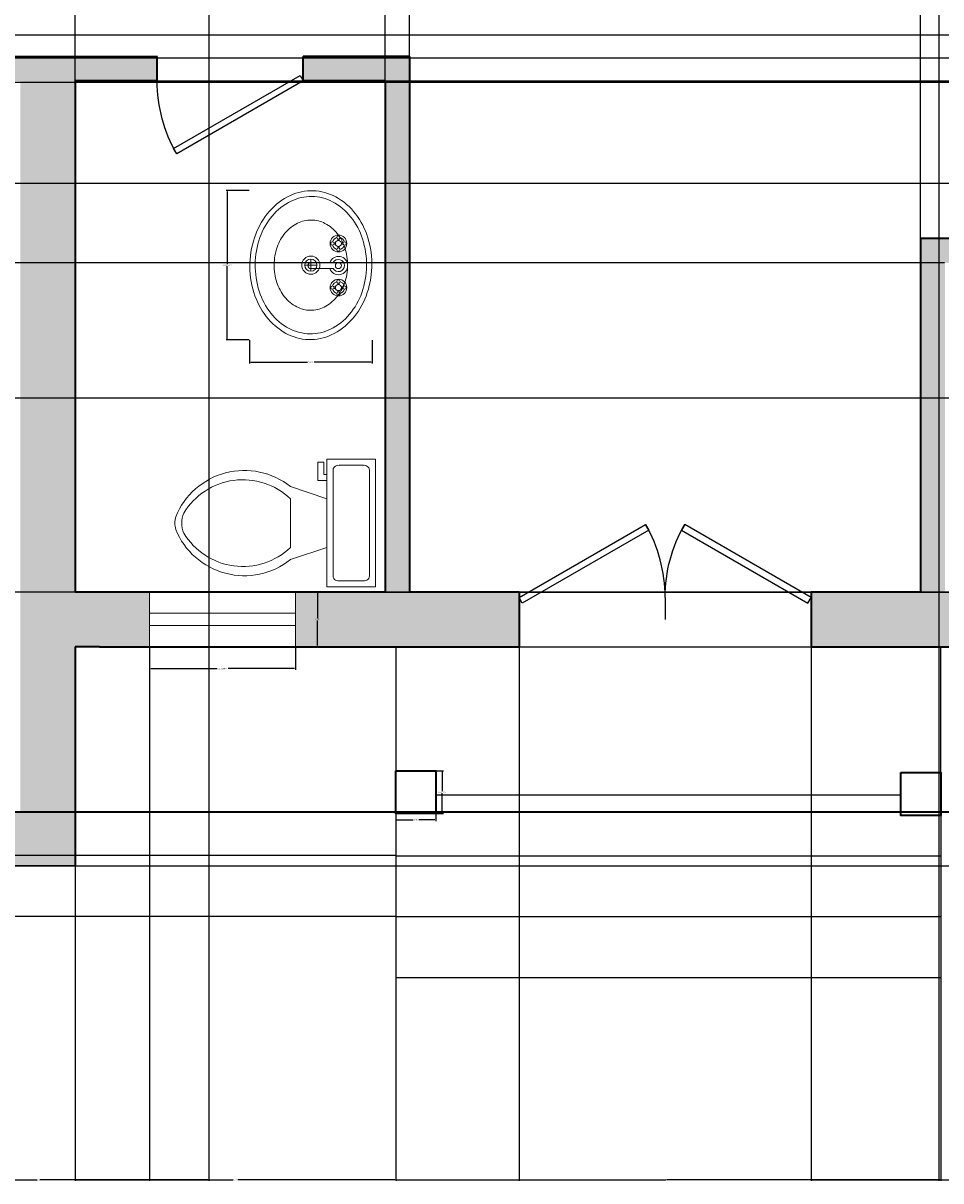
# Model space of a CAD drawing. Units: inches. Extents: x 1531 to 2263, y 2711 to 3216.
# Tile 7 of 12: x 1925 to 2076, y 2711 to 2901. Entities that reach past the tile are written whole.
import ezdxf

# ---------------------------------------------------------------- set-up
doc = ezdxf.new("R2010")
doc.units = ezdxf.units.IN
for name, color, linetype, lineweight in [('A-ANNO-DIMS', 2, 'Continuous', 18), ('A-COLS', 7, 'Continuous', 35), ('A-DOOR', 3, 'Continuous', 25), ('A-FLOR-FIXT', 9, 'Continuous', 18), ('A-FLOR-STRS', 7, 'Continuous', 25), ('A-GLAZ', 4, 'Continuous', 18), ('A-WALL', 7, 'Continuous', 35)]:
    doc.layers.add(name, color=color, linetype=linetype, lineweight=lineweight)
doc.layers.add('A-WALL-PATT', color=18, linetype='Continuous', lineweight=13, true_color=0x000000)
doc.styles.get("Standard").update_dxf_attribs({"font": 'arial.ttf'})
doc.dimstyles.get("Standard").update_dxf_attribs({"dimtxt": 0.18, "dimasz": 0.18, "dimexe": 0.18, "dimexo": 0.0625, "dimgap": 0.09, "dimtad": 0, "dimtih": 1, "dimtoh": 1, "dimdec": 4, "dimzin": 0, "dimdsep": 46, "dimtxsty": 'Standard', "dimcen": 0.09, "dimadec": 0, "dimazin": 0, "dimtfac": 1, "dimtdec": 4, "dimtofl": 0, "dimtmove": 0, "dimatfit": 3, "dimfxl": 1, "dimtolj": 1, "dimtzin": 0, "dimarcsym": 0})

# ---------------------------------------------------------------- blocks, each defined once
blk = doc.blocks.new('*U3')
for p, q in [((0, 0), (0, -6)), ((40, 0), (40, -6))]:
    blk.add_line(p, q)
blk.add_lwpolyline([(0, 0), (34.64, 20), (35.52, 18.48), (0.87, -1.52)], close=True)
blk.add_arc((0, 0), 40, 0, 30)
blk = doc.blocks.new('*U6')
for p, q in [((0, 0), (0, 6)), ((40, 0), (40, 6))]:
    blk.add_line(p, q)
blk.add_lwpolyline([(0, 0), (34.64, -20), (35.52, -18.48), (0.87, 1.52)], close=True)
blk.add_arc((0, 0), 40, 330, 0)
blk = doc.blocks.new('Toilet - top')
for p, q in [((9.5, -6), (9.5, -2)), ((-10, -8.5), (-8, -8.5)), ((-10, -9.5), (-10, -8.5)), ((-7, -9.5), (-10, -9.5)), ((-8, -8.5), (-8, -8)), ((-7, -8), (-7, -9.5)), ((-4, -8), (-6, -14)), ((4, -8), (6, -14)), ((4, -14), (-4, -14))]:
    blk.add_line(p, q)
blk.add_lwpolyline([(10.5, -8), (10.5, 0), (-10.5, 0), (-10.5, -8)], close=True)
for points in [[(8.5, -1), (-8.5, -1)], [(-9.5, -2), (-9.5, -6)], [(-8.5, -7), (8.5, -7)]]:
    blk.add_lwpolyline(points)
for centre, radius, start, end in [((-8.62, -1.88), 0.884, 81.8699, 188.1301), ((8.62, -1.88), 0.884, 351.8699, 98.1301), ((-8.62, -6.12), 0.884, 171.8699, 278.1301), ((8.62, -6.12), 0.884, 261.8699, 8.1301), ((3.52, -21.58), 12.17, 141.4691, 247.9714), ((4.2, -21.82), 11.33, 136.3677, 238.9468), ((-3.52, -21.58), 12.17, 292.0284, 38.5307), ((-4.2, -21.82), 11.33, 301.053, 43.6321), ((0, -27.88), 4, 245.7318, 294.2682), ((0, -29), 4, 254.8605, 285.1395)]:
    blk.add_arc(centre, radius, start, end)
blk = doc.blocks.new('Sink - Oval top')
for p, q in [((-1, 0), (1, 0)), ((0, 1), (0, -1))]:
    blk.add_line(p, q)
for points in [[(-12.23, 0.39, 0.117634), (-11.46, -3.36, 0.104469), (-8.88, -6.8, 0.090016), (-5.08, -9.07, 0.08192), (-0.32, -10.02, 0.08192), (4.49, -9.38, 0.090016), (8.42, -7.36, 0.104469), (11.22, -4.09, 0.117634), (12.23, -0.39, 0.117634), (11.46, 3.36, 0.104469), (8.88, 6.8, 0.090016), (5.08, 9.07, 0.08192), (0.32, 10.02, 0.08192), (-4.49, 9.38, 0.090016), (-8.42, 7.36, 0.104469), (-11.22, 4.09, 0.117634)], [(-11.29, 0.16, 0.118622), (-10.52, -3.25, 0.104678), (-8.07, -6.36, 0.089562), (-4.54, -8.37, 0.081185), (-0.13, -9.15, 0.081185), (4.3, -8.49, 0.089562), (7.89, -6.58, 0.104678), (10.42, -3.55, 0.118622), (11.29, -0.16, 0.118622), (10.52, 3.25, 0.104678), (8.07, 6.36, 0.089562), (4.54, 8.37, 0.081185), (0.13, 9.15, 0.081185), (-4.3, 8.49, 0.089562), (-7.89, 6.58, 0.104678), (-10.42, 3.55, 0.118622)], [(-7.42, 0.08, 0.118283), (-6.91, -2.17, 0.104607), (-5.29, -4.21, 0.089718), (-2.97, -5.53, 0.081436), (-0.07, -6.04, 0.081436), (2.84, -5.59, 0.089718), (5.2, -4.33, 0.104607), (6.86, -2.32, 0.118283), (7.42, -0.08, 0.118283), (6.91, 2.17, 0.104607), (5.29, 4.21, 0.089718), (2.97, 5.53, 0.081436), (0.07, 6.04, 0.081436), (-2.84, 5.59, 0.089718), (-5.2, 4.33, 0.104607), (-6.86, 2.32, 0.118283)]]:
    blk.add_lwpolyline(points, format="xyb", close=True)
for radius in [1.5, 1]:
    blk.add_circle((0, 0), radius)
blk = doc.blocks.new('Faucet - Bathroom top')
for p, q in [((-4.107, 0.125), (-4.375, 0.125)), ((-3.75, 0.4788), (-3.75, 0.75)), ((-3.5, 0.482), (-3.5, 0.75)), ((-3.1461, 0.125), (-2.875, 0.125)), ((3.143, 0.125), (2.875, 0.125)), ((3.5, 0.4788), (3.5, 0.75)), ((3.75, 0.482), (3.75, 0.75)), ((4.1039, 0.125), (4.375, 0.125)), ((-4.1039, -0.125), (-4.375, -0.125)), ((-3.75, -0.4821), (-3.75, -0.75)), ((-3.5, -0.4789), (-3.5, -0.75)), ((-3.143, -0.125), (-2.875, -0.125)), ((-0.5, -0.8639), (-0.5, -4.5)), ((0.5, -4.5), (0.5, -0.8631)), ((3.1461, -0.125), (2.875, -0.125)), ((3.5, -0.4821), (3.5, -0.75)), ((3.75, -0.4789), (3.75, -0.75)), ((4.107, -0.125), (4.375, -0.125))]:
    blk.add_line(p, q)
for centre, radius in [((-3.625, 0), 1.375), ((-4.625, 0), 0.2795), ((-3.625, 0), 0.5), ((-3.625, 1), 0.2795), ((-2.625, 0), 0.2795), ((0, 0), 0.5), ((3.625, 0), 1.375), ((2.625, 0), 0.2795), ((3.625, 0), 0.5), ((3.625, 1), 0.2795), ((4.625, 0), 0.2795), ((-3.625, -1), 0.2795), ((3.625, -1), 0.2795)]:
    blk.add_circle(centre, radius)
for centre, radius, start, end in [((-3.625, 0), 1, 105.2407, 164.2093), ((-3.625, 0), 1, 16.44125, 74.07887), ((0, 0), 1.5, 289.6514, 250.3603), ((0, 0), 1, 300.3431, 239.7554), ((3.625, 0), 1, 106.12, 164.0884), ((3.625, 0), 1, 16.23422, 73.90469), ((-3.625, 0), 1, 196.2342, 253.9047), ((-3.625, 0), 1, 286.12, 344.0884), ((3.625, 0), 1, 196.4413, 254.0789), ((3.625, 0), 1, 285.2407, 344.2093), ((0, -4.5), 0.5, 180, 0)]:
    blk.add_arc(centre, radius, start, end)
blk = doc.blocks.new('WIN-24IN')
for p, q in [((0, 5.5), (24, 5.5)), ((0, 3.5), (24, 3.5))]:
    blk.add_line(p, q)
for points in [[(0, 9), (0, 0)], [(24, 0), (24, 9)]]:
    blk.add_lwpolyline(points)
blk = doc.blocks.new('PORCH-POST')
blk.add_lwpolyline([(0, 7.03), (6.58, 7.03), (6.58, 0), (0, 0)], close=True)
blk = doc.blocks.new('*D28')
at = {"layer": 'A-ANNO-DIMS', "color": 0, "lineweight": -2, "transparency": 16777216}
for p, q in [((1946.17, 2798.8), (1946.17, 2795.08)), ((1970.17, 2798.8), (1970.17, 2795.08)), ((1946.35, 2795.26), (1957.27, 2795.26)), ((1969.99, 2795.26), (1959.06, 2795.26))]:
    blk.add_line(p, q, dxfattribs=at)
at = {"layer": 'A-ANNO-DIMS', "color": 0, "transparency": 16777216}
for points in [[(1946.35, 2795.29), (1946.35, 2795.23), (1946.17, 2795.26)], [(1969.99, 2795.29), (1969.99, 2795.23), (1970.17, 2795.26)]]:
    blk.add_solid(points, dxfattribs=at)
at = {"layer": 'Defpoints', "color": 0, "transparency": 16777216}
for p in [(1946.17, 2798.86), (1970.17, 2798.86), (1970.17, 2795.26)]:
    blk.add_point(p, dxfattribs=at)
at = {"layer": 'A-ANNO-DIMS', "color": 0, "transparency": 16777216, "insert": (1958.17, 2795.26), "char_height": 0.18, "attachment_point": 5}
blk.add_mtext('\\A1;WDW 24 TYP.', dxfattribs=at)
blk = doc.blocks.new('*D29')
at = {"layer": 'A-ANNO-DIMS', "color": 0, "lineweight": -2, "transparency": 16777216}
for p, q in [((1970.23, 2807.86), (1973.95, 2807.86)), ((1973.77, 2807.68), (1973.77, 2803.55)), ((1973.77, 2799.04), (1973.77, 2803.18)), ((1970.23, 2798.86), (1973.95, 2798.86))]:
    blk.add_line(p, q, dxfattribs=at)
at = {"layer": 'A-ANNO-DIMS', "color": 0, "transparency": 16777216}
for points in [[(1973.74, 2807.68), (1973.8, 2807.68), (1973.77, 2807.86)], [(1973.74, 2799.04), (1973.8, 2799.04), (1973.77, 2798.86)]]:
    blk.add_solid(points, dxfattribs=at)
at = {"layer": 'Defpoints', "color": 0, "transparency": 16777216}
for p in [(1970.17, 2807.86), (1973.77, 2807.86), (1970.17, 2798.86)]:
    blk.add_point(p, dxfattribs=at)
at = {"layer": 'A-ANNO-DIMS', "color": 0, "transparency": 16777216, "insert": (1973.77, 2803.36), "char_height": 0.18, "attachment_point": 5}
blk.add_mtext('\\A1;9 TYP.', dxfattribs=at)
blk = doc.blocks.new('*D38')
at = {"layer": 'A-ANNO-DIMS', "color": 0, "lineweight": -2, "transparency": 16777216}
for p, q in [((1962.54, 2873.87), (1958.74, 2873.87)), ((1958.92, 2873.69), (1958.92, 2861.78)), ((1958.92, 2849.5), (1958.92, 2861.41)), ((1962.54, 2849.32), (1958.74, 2849.32))]:
    blk.add_line(p, q, dxfattribs=at)
at = {"layer": 'A-ANNO-DIMS', "color": 0, "transparency": 16777216}
for points in [[(1958.89, 2873.69), (1958.95, 2873.69), (1958.92, 2873.87)], [(1958.89, 2849.5), (1958.95, 2849.5), (1958.92, 2849.32)]]:
    blk.add_solid(points, dxfattribs=at)
at = {"layer": 'Defpoints', "color": 0, "transparency": 16777216}
for p in [(1962.6, 2873.87), (1958.92, 2849.32), (1962.6, 2849.32)]:
    blk.add_point(p, dxfattribs=at)
at = {"layer": 'A-ANNO-DIMS', "color": 0, "transparency": 16777216, "insert": (1958.92, 2861.59), "char_height": 0.18, "attachment_point": 5}
blk.add_mtext('\\A1;BASIN 25 TYP.', dxfattribs=at)
blk = doc.blocks.new('*D39')
at = {"layer": 'A-ANNO-DIMS', "color": 0, "lineweight": -2, "transparency": 16777216}
for p, q in [((1962.6, 2849.25), (1962.6, 2845.45)), ((1982.74, 2849.25), (1982.74, 2845.45)), ((1962.78, 2845.63), (1972.14, 2845.63)), ((1982.56, 2845.63), (1973.2, 2845.63))]:
    blk.add_line(p, q, dxfattribs=at)
at = {"layer": 'A-ANNO-DIMS', "color": 0, "transparency": 16777216}
for points in [[(1962.78, 2845.66), (1962.78, 2845.6), (1962.6, 2845.63)], [(1982.56, 2845.66), (1982.56, 2845.6), (1982.74, 2845.63)]]:
    blk.add_solid(points, dxfattribs=at)
at = {"layer": 'Defpoints', "color": 0, "transparency": 16777216}
for p in [(1962.6, 2849.32), (1982.74, 2849.32), (1982.74, 2845.63)]:
    blk.add_point(p, dxfattribs=at)
at = {"layer": 'A-ANNO-DIMS', "color": 0, "transparency": 16777216, "insert": (1972.67, 2845.63), "char_height": 0.18, "attachment_point": 5}
blk.add_mtext('\\A1;20 TYP.', dxfattribs=at)
blk = doc.blocks.new('*D44')
at = {"layer": 'A-ANNO-DIMS', "color": 0, "lineweight": -2, "transparency": 16777216}
for p, q in [((1993.29, 2778.47), (1994.46, 2778.47)), ((1994.28, 2778.29), (1994.28, 2775.14)), ((1994.28, 2771.62), (1994.28, 2774.77)), ((1993.29, 2771.44), (1994.46, 2771.44))]:
    blk.add_line(p, q, dxfattribs=at)
at = {"layer": 'A-ANNO-DIMS', "color": 0, "transparency": 16777216}
for points in [[(1994.25, 2778.29), (1994.31, 2778.29), (1994.28, 2778.47)], [(1994.25, 2771.62), (1994.31, 2771.62), (1994.28, 2771.44)]]:
    blk.add_solid(points, dxfattribs=at)
at = {"layer": 'Defpoints', "color": 0, "transparency": 16777216}
for p in [(1993.23, 2778.47), (1994.28, 2778.47), (1993.23, 2771.44)]:
    blk.add_point(p, dxfattribs=at)
at = {"layer": 'A-ANNO-DIMS', "color": 0, "transparency": 16777216, "insert": (1994.28, 2774.96), "char_height": 0.18, "attachment_point": 5}
blk.add_mtext('\\A1;POST 7 TYP.', dxfattribs=at)
blk = doc.blocks.new('*D45')
at = {"layer": 'A-ANNO-DIMS', "color": 0, "lineweight": -2, "transparency": 16777216}
for p, q in [((1986.65, 2771.38), (1986.65, 2770.2)), ((1993.23, 2771.38), (1993.23, 2770.2)), ((1986.83, 2770.38), (1989.48, 2770.38)), ((1993.05, 2770.38), (1990.4, 2770.38))]:
    blk.add_line(p, q, dxfattribs=at)
at = {"layer": 'A-ANNO-DIMS', "color": 0, "transparency": 16777216}
for points in [[(1986.83, 2770.41), (1986.83, 2770.35), (1986.65, 2770.38)], [(1993.05, 2770.41), (1993.05, 2770.35), (1993.23, 2770.38)]]:
    blk.add_solid(points, dxfattribs=at)
at = {"layer": 'Defpoints', "color": 0, "transparency": 16777216}
for p in [(1986.65, 2771.44), (1993.23, 2771.44), (1993.23, 2770.38)]:
    blk.add_point(p, dxfattribs=at)
at = {"layer": 'A-ANNO-DIMS', "color": 0, "transparency": 16777216, "insert": (1989.94, 2770.38), "char_height": 0.18, "attachment_point": 5}
blk.add_mtext('\\A1;7 TYP.', dxfattribs=at)
blk = doc.blocks.new('*D60')
at = {"layer": 'A-ANNO-DIMS', "color": 0, "lineweight": -2, "transparency": 16777216}
for p, q in [((1899.91, 3097.79), (1899.91, 2711.06)), ((1955.91, 3097.81), (1955.91, 2711.06)), ((1900.09, 2711.24), (1927.69, 2711.24)), ((1955.73, 2711.24), (1928.13, 2711.24))]:
    blk.add_line(p, q, dxfattribs=at)
at = {"layer": 'A-ANNO-DIMS', "color": 0, "transparency": 16777216}
for points in [[(1900.09, 2711.27), (1900.09, 2711.21), (1899.91, 2711.24)], [(1955.73, 2711.27), (1955.73, 2711.21), (1955.91, 2711.24)]]:
    blk.add_solid(points, dxfattribs=at)
at = {"layer": 'Defpoints', "color": 0, "transparency": 16777216}
for p in [(1899.91, 3097.85), (1955.91, 3097.88), (1955.91, 2711.24)]:
    blk.add_point(p, dxfattribs=at)
at = {"layer": 'A-ANNO-DIMS', "color": 0, "transparency": 16777216, "insert": (1927.91, 2711.24), "char_height": 0.18, "attachment_point": 5}
blk.add_mtext('\\A1;56', dxfattribs=at)
blk = doc.blocks.new('*D65')
at = {"layer": 'A-ANNO-DIMS', "color": 0, "lineweight": -2, "transparency": 16777216}
for p, q in [((1577.97, 2891.68), (2262.37, 2891.68)), ((2262.19, 2891.5), (2262.19, 2831.86)), ((2262.19, 2771.86), (2262.19, 2831.5)), ((1577.97, 2771.68), (2262.37, 2771.68))]:
    blk.add_line(p, q, dxfattribs=at)
at = {"layer": 'A-ANNO-DIMS', "color": 0, "transparency": 16777216}
for points in [[(2262.16, 2891.5), (2262.22, 2891.5), (2262.19, 2891.68)], [(2262.16, 2771.86), (2262.22, 2771.86), (2262.19, 2771.68)]]:
    blk.add_solid(points, dxfattribs=at)
at = {"layer": 'Defpoints', "color": 0, "transparency": 16777216}
for p in [(1577.91, 2891.68), (1577.91, 2771.68), (2262.19, 2771.68)]:
    blk.add_point(p, dxfattribs=at)
at = {"layer": 'A-ANNO-DIMS', "color": 0, "transparency": 16777216, "insert": (2262.19, 2831.68), "char_height": 0.18, "attachment_point": 5}
blk.add_mtext('\\A1;120', dxfattribs=at)
blk = doc.blocks.new('*D70')
at = {"layer": 'A-ANNO-DIMS', "color": 0, "lineweight": -2, "transparency": 16777216}
for p, q in [((1736.97, 2839.76), (2262.37, 2839.76)), ((2262.19, 2839.58), (2262.19, 2805.94)), ((2262.19, 2771.94), (2262.19, 2805.58)), ((1736.97, 2771.76), (2262.37, 2771.76))]:
    blk.add_line(p, q, dxfattribs=at)
at = {"layer": 'A-ANNO-DIMS', "color": 0, "transparency": 16777216}
for points in [[(2262.16, 2839.58), (2262.22, 2839.58), (2262.19, 2839.76)], [(2262.16, 2771.94), (2262.22, 2771.94), (2262.19, 2771.76)]]:
    blk.add_solid(points, dxfattribs=at)
at = {"layer": 'Defpoints', "color": 0, "transparency": 16777216}
for p in [(1736.91, 2839.76), (2262.19, 2839.76), (1736.91, 2771.76)]:
    blk.add_point(p, dxfattribs=at)
at = {"layer": 'A-ANNO-DIMS', "color": 0, "transparency": 16777216, "insert": (2262.19, 2805.76), "char_height": 0.18, "attachment_point": 5}
blk.add_mtext('\\A1;68', dxfattribs=at)
blk = doc.blocks.new('*D71')
at = {"layer": 'A-ANNO-DIMS', "color": 0, "lineweight": -2, "transparency": 16777216}
for p, q in [((1933.91, 2891.93), (1933.91, 3216.47)), ((1934.09, 3216.29), (1959.21, 3216.29)), ((1984.73, 3216.29), (1959.61, 3216.29)), ((1984.91, 2891.95), (1984.91, 3216.47))]:
    blk.add_line(p, q, dxfattribs=at)
at = {"layer": 'A-ANNO-DIMS', "color": 0, "transparency": 16777216}
for points in [[(1934.09, 3216.32), (1934.09, 3216.26), (1933.91, 3216.29)], [(1984.73, 3216.32), (1984.73, 3216.26), (1984.91, 3216.29)]]:
    blk.add_solid(points, dxfattribs=at)
at = {"layer": 'Defpoints', "color": 0, "transparency": 16777216}
for p in [(1984.91, 3216.29), (1933.91, 2891.87), (1984.91, 2891.89)]:
    blk.add_point(p, dxfattribs=at)
at = {"layer": 'A-ANNO-DIMS', "color": 0, "transparency": 16777216, "insert": (1959.41, 3216.29), "char_height": 0.18, "attachment_point": 5}
blk.add_mtext('\\A1;51', dxfattribs=at)
blk = doc.blocks.new('*D72')
at = {"layer": 'A-ANNO-DIMS', "color": 0, "lineweight": -2, "transparency": 16777216}
for p, q in [((1986.65, 2744.45), (1986.65, 2711.06)), ((2076.24, 2744.45), (2076.24, 2711.06)), ((1986.83, 2711.24), (2031.05, 2711.24)), ((2076.06, 2711.24), (2031.84, 2711.24))]:
    blk.add_line(p, q, dxfattribs=at)
at = {"layer": 'A-ANNO-DIMS', "color": 0, "transparency": 16777216}
for points in [[(1986.83, 2711.27), (1986.83, 2711.21), (1986.65, 2711.24)], [(2076.06, 2711.27), (2076.06, 2711.21), (2076.24, 2711.24)]]:
    blk.add_solid(points, dxfattribs=at)
at = {"layer": 'Defpoints', "color": 0, "transparency": 16777216}
for p in [(1986.65, 2744.52), (2076.24, 2744.52), (2076.24, 2711.24)]:
    blk.add_point(p, dxfattribs=at)
at = {"layer": 'A-ANNO-DIMS', "color": 0, "transparency": 16777216, "insert": (2031.44, 2711.24), "char_height": 0.18, "attachment_point": 5}
blk.add_mtext('\\A1;89.59', dxfattribs=at)
blk = doc.blocks.new('*D75')
at = {"layer": 'A-ANNO-DIMS', "color": 0, "lineweight": -2, "transparency": 16777216}
for p, q in [((2219.85, 2899.4), (1531.04, 2899.4)), ((1531.22, 2899.22), (1531.22, 2853.81)), ((1531.22, 2808.04), (1531.22, 2853.45)), ((2219.85, 2807.86), (1531.04, 2807.86))]:
    blk.add_line(p, q, dxfattribs=at)
at = {"layer": 'A-ANNO-DIMS', "color": 0, "transparency": 16777216}
for points in [[(1531.19, 2899.22), (1531.25, 2899.22), (1531.22, 2899.4)], [(1531.19, 2808.04), (1531.25, 2808.04), (1531.22, 2807.86)]]:
    blk.add_solid(points, dxfattribs=at)
at = {"layer": 'Defpoints', "color": 0, "transparency": 16777216}
for p in [(1531.22, 2899.4), (2219.91, 2899.4), (2219.91, 2807.86)]:
    blk.add_point(p, dxfattribs=at)
at = {"layer": 'A-ANNO-DIMS', "color": 0, "transparency": 16777216, "insert": (1531.22, 2853.63), "char_height": 0.18, "attachment_point": 5}
blk.add_mtext('\\A1;91.53', dxfattribs=at)
blk = doc.blocks.new('*D78')
at = {"layer": 'A-ANNO-DIMS', "color": 0, "lineweight": -2, "transparency": 16777216}
for p, q in [((2006.91, 2798.8), (2006.91, 2711.06)), ((2054.91, 2798.8), (2054.91, 2711.06)), ((2007.09, 2711.24), (2030.69, 2711.24)), ((2054.73, 2711.24), (2031.13, 2711.24))]:
    blk.add_line(p, q, dxfattribs=at)
at = {"layer": 'A-ANNO-DIMS', "color": 0, "transparency": 16777216}
for points in [[(2007.09, 2711.27), (2007.09, 2711.21), (2006.91, 2711.24)], [(2054.73, 2711.27), (2054.73, 2711.21), (2054.91, 2711.24)]]:
    blk.add_solid(points, dxfattribs=at)
at = {"layer": 'Defpoints', "color": 0, "transparency": 16777216}
for p in [(2006.91, 2798.86), (2054.91, 2798.86), (2054.91, 2711.24)]:
    blk.add_point(p, dxfattribs=at)
at = {"layer": 'A-ANNO-DIMS', "color": 0, "transparency": 16777216, "insert": (2030.91, 2711.24), "char_height": 0.18, "attachment_point": 5}
blk.add_mtext('\\A1;48', dxfattribs=at)
blk = doc.blocks.new('*D79')
at = {"layer": 'A-ANNO-DIMS', "color": 0, "lineweight": -2, "transparency": 16777216}
for p, q in [((1988.91, 2807.93), (1988.91, 3216.47)), ((1989.09, 3216.29), (2030.69, 3216.29)), ((2072.73, 3216.29), (2031.13, 3216.29)), ((2072.91, 2807.93), (2072.91, 3216.47))]:
    blk.add_line(p, q, dxfattribs=at)
at = {"layer": 'A-ANNO-DIMS', "color": 0, "transparency": 16777216}
for points in [[(1989.09, 3216.32), (1989.09, 3216.26), (1988.91, 3216.29)], [(2072.73, 3216.32), (2072.73, 3216.26), (2072.91, 3216.29)]]:
    blk.add_solid(points, dxfattribs=at)
at = {"layer": 'Defpoints', "color": 0, "transparency": 16777216}
for p in [(2072.91, 3216.29), (1988.91, 2807.86), (2072.91, 2807.86)]:
    blk.add_point(p, dxfattribs=at)
at = {"layer": 'A-ANNO-DIMS', "color": 0, "transparency": 16777216, "insert": (2030.91, 3216.29), "char_height": 0.18, "attachment_point": 5}
blk.add_mtext('\\A1;84', dxfattribs=at)
blk = doc.blocks.new('*D81')
at = {"layer": 'A-ANNO-DIMS', "color": 0, "lineweight": -2, "transparency": 16777216}
for p, q in [((1933.97, 2891.87), (2262.37, 2891.87)), ((2262.19, 2891.69), (2262.19, 2850.05)), ((2262.19, 2808.04), (2262.19, 2849.68)), ((1933.97, 2807.86), (2262.37, 2807.86))]:
    blk.add_line(p, q, dxfattribs=at)
at = {"layer": 'A-ANNO-DIMS', "color": 0, "transparency": 16777216}
for points in [[(2262.16, 2891.69), (2262.22, 2891.69), (2262.19, 2891.87)], [(2262.16, 2808.04), (2262.22, 2808.04), (2262.19, 2807.86)]]:
    blk.add_solid(points, dxfattribs=at)
at = {"layer": 'Defpoints', "color": 0, "transparency": 16777216}
for p in [(1933.91, 2891.87), (2262.19, 2891.87), (1933.91, 2807.86)]:
    blk.add_point(p, dxfattribs=at)
at = {"layer": 'A-ANNO-DIMS', "color": 0, "transparency": 16777216, "insert": (2262.19, 2849.86), "char_height": 0.18, "attachment_point": 5}
blk.add_mtext('\\A1;84', dxfattribs=at)
blk = doc.blocks.new('*D96')
at = {"layer": 'A-ANNO-DIMS', "color": 0, "lineweight": -2, "transparency": 16777216}
for p, q in [((1933.91, 2798.8), (1933.91, 2711.06)), ((1946.17, 2798.8), (1946.17, 2711.06)), ((1934.09, 2711.24), (1939.58, 2711.24)), ((1945.99, 2711.24), (1940.49, 2711.24))]:
    blk.add_line(p, q, dxfattribs=at)
at = {"layer": 'A-ANNO-DIMS', "color": 0, "transparency": 16777216}
for points in [[(1934.09, 2711.27), (1934.09, 2711.21), (1933.91, 2711.24)], [(1945.99, 2711.27), (1945.99, 2711.21), (1946.17, 2711.24)]]:
    blk.add_solid(points, dxfattribs=at)
at = {"layer": 'Defpoints', "color": 0, "transparency": 16777216}
for p in [(1933.91, 2798.86), (1946.17, 2798.86), (1946.17, 2711.24)]:
    blk.add_point(p, dxfattribs=at)
at = {"layer": 'A-ANNO-DIMS', "color": 0, "transparency": 16777216, "insert": (1940.04, 2711.24), "char_height": 0.18, "attachment_point": 5}
blk.add_mtext('\\A1;12.257', dxfattribs=at)
blk = doc.blocks.new('*D97')
at = {"layer": 'A-ANNO-DIMS', "color": 0, "lineweight": -2, "transparency": 16777216}
for p, q in [((2054.91, 2798.8), (2054.91, 2711.06)), ((2121.28, 2798.8), (2121.28, 2711.06)), ((2055.09, 2711.24), (2087.7, 2711.24)), ((2121.09, 2711.24), (2088.49, 2711.24))]:
    blk.add_line(p, q, dxfattribs=at)
at = {"layer": 'A-ANNO-DIMS', "color": 0, "transparency": 16777216}
for points in [[(2055.09, 2711.27), (2055.09, 2711.21), (2054.91, 2711.24)], [(2121.09, 2711.27), (2121.09, 2711.21), (2121.28, 2711.24)]]:
    blk.add_solid(points, dxfattribs=at)
at = {"layer": 'Defpoints', "color": 0, "transparency": 16777216}
for p in [(2054.91, 2798.86), (2121.28, 2798.86), (2054.91, 2711.24)]:
    blk.add_point(p, dxfattribs=at)
at = {"layer": 'A-ANNO-DIMS', "color": 0, "transparency": 16777216, "insert": (2088.09, 2711.24), "char_height": 0.18, "attachment_point": 5}
blk.add_mtext('\\A1;66.36', dxfattribs=at)
blk = doc.blocks.new('*D101')
at = {"layer": 'A-ANNO-DIMS', "color": 0, "lineweight": -2, "transparency": 16777216}
for p, q in [((2228.85, 2918.81), (1531.04, 2918.81)), ((1531.22, 2918.63), (1531.22, 2897.08)), ((1531.22, 2875.18), (1531.22, 2896.72)), ((2228.85, 2875), (1531.04, 2875))]:
    blk.add_line(p, q, dxfattribs=at)
at = {"layer": 'A-ANNO-DIMS', "color": 0, "transparency": 16777216}
for points in [[(1531.19, 2918.63), (1531.25, 2918.63), (1531.22, 2918.81)], [(1531.19, 2875.18), (1531.25, 2875.18), (1531.22, 2875)]]:
    blk.add_solid(points, dxfattribs=at)
at = {"layer": 'Defpoints', "color": 0, "transparency": 16777216}
for p in [(2228.91, 2918.81), (1531.22, 2875), (2228.91, 2875)]:
    blk.add_point(p, dxfattribs=at)
at = {"layer": 'A-ANNO-DIMS', "color": 0, "transparency": 16777216, "insert": (1531.22, 2896.9), "char_height": 0.18, "attachment_point": 5}
blk.add_mtext('\\A1;43.81', dxfattribs=at)
blk = doc.blocks.new('*D108')
at = {"layer": 'A-ANNO-DIMS', "color": 0, "lineweight": -2, "transparency": 16777216}
for p, q in [((1933.97, 2798.86), (2262.37, 2798.86)), ((2262.19, 2798.68), (2262.19, 2781.05)), ((2262.19, 2763.05), (2262.19, 2780.68)), ((1933.97, 2762.87), (2262.37, 2762.87))]:
    blk.add_line(p, q, dxfattribs=at)
at = {"layer": 'A-ANNO-DIMS', "color": 0, "transparency": 16777216}
for points in [[(2262.16, 2798.68), (2262.22, 2798.68), (2262.19, 2798.86)], [(2262.16, 2763.05), (2262.22, 2763.05), (2262.19, 2762.87)]]:
    blk.add_solid(points, dxfattribs=at)
at = {"layer": 'Defpoints', "color": 0, "transparency": 16777216}
for p in [(1933.91, 2798.86), (2262.19, 2798.86), (1933.91, 2762.87)]:
    blk.add_point(p, dxfattribs=at)
at = {"layer": 'A-ANNO-DIMS', "color": 0, "transparency": 16777216, "insert": (2262.19, 2780.86), "char_height": 0.18, "attachment_point": 5}
blk.add_mtext('\\A1;36', dxfattribs=at)
blk = doc.blocks.new('*D109')
at = {"layer": 'A-ANNO-DIMS', "color": 0, "lineweight": -2, "transparency": 16777216}
for p, q in [((1933.91, 2798.8), (1933.91, 2711.06)), ((1986.65, 2798.8), (1986.65, 2711.06)), ((1934.09, 2711.24), (1959.89, 2711.24)), ((1986.47, 2711.24), (1960.67, 2711.24))]:
    blk.add_line(p, q, dxfattribs=at)
at = {"layer": 'A-ANNO-DIMS', "color": 0, "transparency": 16777216}
for points in [[(1934.09, 2711.27), (1934.09, 2711.21), (1933.91, 2711.24)], [(1986.47, 2711.27), (1986.47, 2711.21), (1986.65, 2711.24)]]:
    blk.add_solid(points, dxfattribs=at)
at = {"layer": 'Defpoints', "color": 0, "transparency": 16777216}
for p in [(1933.91, 2798.86), (1986.65, 2798.86), (1986.65, 2711.24)]:
    blk.add_point(p, dxfattribs=at)
at = {"layer": 'A-ANNO-DIMS', "color": 0, "transparency": 16777216, "insert": (1960.28, 2711.24), "char_height": 0.18, "attachment_point": 5}
blk.add_mtext('\\A1;52.74', dxfattribs=at)
blk = doc.blocks.new('*D114')
at = {"layer": 'A-ANNO-DIMS', "color": 0, "lineweight": -2, "transparency": 16777216}
for p, q in [((1577.97, 2913.94), (2262.37, 2913.94)), ((2262.19, 2913.76), (2262.19, 2904.99)), ((2262.19, 2895.86), (2262.19, 2904.63)), ((1577.97, 2895.68), (2262.37, 2895.68))]:
    blk.add_line(p, q, dxfattribs=at)
at = {"layer": 'A-ANNO-DIMS', "color": 0, "transparency": 16777216}
for points in [[(2262.16, 2913.76), (2262.22, 2913.76), (2262.19, 2913.94)], [(2262.16, 2895.86), (2262.22, 2895.86), (2262.19, 2895.68)]]:
    blk.add_solid(points, dxfattribs=at)
at = {"layer": 'Defpoints', "color": 0, "transparency": 16777216}
for p in [(1577.91, 2913.94), (1577.91, 2895.68), (2262.19, 2895.68)]:
    blk.add_point(p, dxfattribs=at)
at = {"layer": 'A-ANNO-DIMS', "color": 0, "transparency": 16777216, "insert": (2262.19, 2904.81), "char_height": 0.18, "attachment_point": 5}
blk.add_mtext('\\A1;18.26', dxfattribs=at)
blk = doc.blocks.new('*D125')
at = {"layer": 'A-ANNO-DIMS', "color": 0, "lineweight": -2, "transparency": 16777216}
for p, q in [((2076.85, 2861.95), (1531.04, 2861.95)), ((1531.22, 2861.77), (1531.22, 2835.09)), ((1531.22, 2808.04), (1531.22, 2834.72)), ((2076.85, 2807.86), (1531.04, 2807.86))]:
    blk.add_line(p, q, dxfattribs=at)
at = {"layer": 'A-ANNO-DIMS', "color": 0, "transparency": 16777216}
for points in [[(1531.19, 2861.77), (1531.25, 2861.77), (1531.22, 2861.95)], [(1531.19, 2808.04), (1531.25, 2808.04), (1531.22, 2807.86)]]:
    blk.add_solid(points, dxfattribs=at)
at = {"layer": 'Defpoints', "color": 0, "transparency": 16777216}
for p in [(2076.91, 2861.95), (1531.22, 2807.86), (2076.91, 2807.86)]:
    blk.add_point(p, dxfattribs=at)
at = {"layer": 'A-ANNO-DIMS', "color": 0, "transparency": 16777216, "insert": (1531.22, 2834.91), "char_height": 0.18, "attachment_point": 5}
blk.add_mtext('\\A1;54.09', dxfattribs=at)
blk = doc.blocks.new('*D130')
at = {"layer": 'A-ANNO-DIMS', "color": 0, "lineweight": -2, "transparency": 16777216}
for p, q in [((2075.91, 3029.88), (2075.91, 2711.06)), ((2079.91, 3025.88), (2079.91, 2711.06)), ((2076.09, 2711.24), (2077.76, 2711.24)), ((2079.73, 2711.24), (2078.06, 2711.24))]:
    blk.add_line(p, q, dxfattribs=at)
at = {"layer": 'A-ANNO-DIMS', "color": 0, "transparency": 16777216}
for points in [[(2076.09, 2711.27), (2076.09, 2711.21), (2075.91, 2711.24)], [(2079.73, 2711.27), (2079.73, 2711.21), (2079.91, 2711.24)]]:
    blk.add_solid(points, dxfattribs=at)
at = {"layer": 'Defpoints', "color": 0, "transparency": 16777216}
for p in [(2075.91, 3029.94), (2079.91, 3025.94), (2075.91, 2711.24)]:
    blk.add_point(p, dxfattribs=at)
at = {"layer": 'A-ANNO-DIMS', "color": 0, "transparency": 16777216, "insert": (2077.91, 2711.24), "char_height": 0.18, "attachment_point": 5}
blk.add_mtext('\\A1;4', dxfattribs=at)
blk = doc.blocks.new('*D131')
at = {"layer": 'A-ANNO-DIMS', "color": 0, "lineweight": -2, "transparency": 16777216}
for p, q in [((1986.59, 2764.52), (1531.04, 2764.52)), ((1531.22, 2764.34), (1531.22, 2759.7)), ((1531.22, 2754.7), (1531.22, 2759.33)), ((1986.59, 2754.52), (1531.04, 2754.52))]:
    blk.add_line(p, q, dxfattribs=at)
at = {"layer": 'A-ANNO-DIMS', "color": 0, "transparency": 16777216}
for points in [[(1531.19, 2764.34), (1531.25, 2764.34), (1531.22, 2764.52)], [(1531.19, 2754.7), (1531.25, 2754.7), (1531.22, 2754.52)]]:
    blk.add_solid(points, dxfattribs=at)
at = {"layer": 'Defpoints', "color": 0, "transparency": 16777216}
for p in [(1531.22, 2764.52), (1986.65, 2764.52), (1986.65, 2754.52)]:
    blk.add_point(p, dxfattribs=at)
at = {"layer": 'A-ANNO-DIMS', "color": 0, "transparency": 16777216, "insert": (1531.22, 2759.52), "char_height": 0.18, "attachment_point": 5}
blk.add_mtext('\\A1;10', dxfattribs=at)

msp = doc.modelspace()

# ---------------------------------------------------------------- hatches: boundary and pattern name
at = {"layer": 'A-WALL-PATT'}
h = msp.add_hatch(color=256, dxfattribs=at)
h.dxf.hatch_style = 1
h.paths.add_polyline_path([(1946.1667, 2807.8631), (1933.9101, 2807.8631), (1933.9101, 2891.8657), (1947.4101, 2891.8728), (1947.4101, 2895.4791), (1947.4101, 2895.8728), (1918.9101, 2895.8579), (1918.9101, 2891.861), (1924.9101, 2891.861), (1924.9101, 2771.8496), (1906.2623, 2771.8496), (1906.2623, 2762.8513), (1933.9101, 2762.8657), (1933.9101, 2771.861), (1933.9101, 2798.8631), (1937.9101, 2798.8631), (1946.1667, 2798.8631)])
h = msp.add_hatch(color=256, dxfattribs=at)
h.dxf.hatch_style = 1
h.paths.add_polyline_path([(2006.9101, 2807.8631), (1988.9101, 2807.8631), (1988.9101, 2895.8945), (1971.4101, 2895.8854), (1971.4101, 2891.8854), (1984.9101, 2891.8924), (1984.9101, 2807.8631), (1970.1667, 2807.8631), (1970.1667, 2798.8631), (2006.9101, 2798.8631)])
h = msp.add_hatch(color=256, dxfattribs=at)
h.dxf.hatch_style = 1
h.paths.add_polyline_path([(2121.275, 2807.8631), (2076.9101, 2807.8631), (2076.9101, 2861.9499), (2098.9101, 2861.9499), (2098.9101, 2869.3336), (2094.9101, 2869.3336), (2094.9101, 2865.9499), (2072.9101, 2865.9499), (2072.9101, 2807.8631), (2054.9101, 2807.8631), (2054.9101, 2798.8631), (2121.275, 2798.8631)])

# ---------------------------------------------------------------- linework, layer by layer
at = {"layer": 'A-FLOR-STRS'}
for p, q in [((1986.6484, 2798.8631), (1986.6484, 2774.5157)), ((2076.2365, 2774.5157), (2076.2365, 2798.8631)), ((1986.6484, 2774.5157), (1986.6484, 2744.5157)), ((1993.2285, 2774.5157), (2069.6564, 2774.5157)), ((2076.2365, 2774.5157), (2076.2365, 2744.5157)), ((1986.6484, 2764.5157), (2070.4922, 2764.5157)), ((2070.4922, 2764.5157), (2076.2365, 2764.5157)), ((1986.6484, 2754.5157), (2070.4922, 2754.5157)), ((2070.4922, 2754.5157), (2076.2365, 2754.5157)), ((1986.6484, 2744.5157), (2070.4922, 2744.5157)), ((2070.4922, 2744.5157), (2076.2365, 2744.5157))]:
    msp.add_line(p, q, dxfattribs=at)
at = {"layer": 'A-WALL'}
for p, q in [((1947.4101, 2895.8728), (1918.9101, 2895.8579)), ((1947.4101, 2891.8728), (1947.4101, 2895.8791)), ((1988.9101, 2895.8945), (1971.4101, 2895.8854)), ((1971.4101, 2891.8791), (1971.4101, 2895.8854)), ((1988.9101, 2895.8945), (1988.9101, 2807.8631)), ((1947.4101, 2891.8728), (1933.9101, 2891.8657)), ((1933.9101, 2891.8657), (1933.9101, 2807.8631)), ((1984.9101, 2891.8924), (1971.4101, 2891.8854)), ((1984.9101, 2891.8924), (1984.9101, 2807.8631)), ((2072.9101, 2865.9499), (2072.9101, 2807.8631)), ((2094.9258, 2865.9499), (2072.9101, 2865.9499)), ((1933.9101, 2807.8631), (1984.9101, 2807.8631)), ((1988.9101, 2807.8631), (2006.9101, 2807.8631)), ((2006.9101, 2807.8631), (2006.9101, 2798.8631)), ((2054.9101, 2807.8631), (2054.9101, 2798.8631)), ((2054.9101, 2807.8631), (2072.9101, 2807.8631)), ((1937.9101, 2798.8631), (1933.9101, 2798.8631)), ((1933.9101, 2798.8631), (1933.9101, 2771.861)), ((1937.9101, 2798.8631), (2006.9101, 2798.8631)), ((2054.9101, 2798.8631), (2228.9101, 2798.8631)), ((1933.9101, 2771.861), (1933.9101, 2762.8657))]:
    msp.add_line(p, q, dxfattribs=at)
msp.add_lwpolyline([(1933.9101, 2762.8657), (1568.9111, 2762.6748), (1568.9111, 3182.6749), (2228.9101, 3183.02), (2228.9101, 2798.8631)], dxfattribs=at)

# ---------------------------------------------------------------- block references
at = {"layer": 'A-COLS'}
for p in [(1986.648, 2771.438), (2069.656, 2771.1367)]:
    msp.add_blockref('PORCH-POST', p, dxfattribs=at)
at = {"layer": 'A-DOOR', "yscale": 0.6, "zscale": 0.6}
for name, p, xscale in [('*U6', (1971.4101, 2891.8791), -0.6), ('*U3', (2006.9101, 2806.9631), 0.6), ('*U3', (2054.9101, 2806.9631), -0.6)]:
    msp.add_blockref(name, p, dxfattribs=dict(at, xscale=xscale))
at = {"layer": 'A-FLOR-FIXT', "rotation": 270}
for name, p in [('Sink - Oval top', (1972.6719, 2861.5922)), ('Faucet - Bathroom top', (1977.2087, 2861.5245)), ('Toilet - top', (1983.3156, 2819.1869))]:
    msp.add_blockref(name, p, dxfattribs=at)
at = {"layer": 'A-GLAZ'}
msp.add_blockref('WIN-24IN', (1946.167, 2798.8628), dxfattribs=at)

# ---------------------------------------------------------------- dimensions: what is measured, and where the dimension line sits
at = {"layer": 'A-ANNO-DIMS'}
for base, p1, p2, override, picture, middle in [((1984.9101, 3216.295), (1933.9101, 2891.8657), (1984.9101, 2891.8924), {"dimdec": 0, "dimlfac": 1, "dimrnd": 0, "dimzin": 0, "dimdsep": 46, "dimlunit": 2}, '*D71', (1959.4101, 3216.295)), ((2072.9101, 3216.295), (1988.9101, 2807.8631), (2072.9101, 2807.8631), {"dimdec": 0, "dimlfac": 1, "dimrnd": 0, "dimzin": 0, "dimdsep": 46, "dimlunit": 2}, '*D79', (2030.9101, 3216.295)), ((1955.9101, 2711.2407), (1899.9101, 3097.8479), (1955.9101, 3097.8772), {"dimdec": 0, "dimlfac": 1, "dimrnd": 0, "dimzin": 0, "dimdsep": 46, "dimlunit": 2}, '*D60', (1927.9101, 2711.2407)), ((2075.9101, 2711.2407), (2079.9101, 3025.9421), (2075.9101, 3029.94), {"dimdec": 0, "dimlfac": 1, "dimrnd": 0, "dimzin": 0, "dimdsep": 46, "dimlunit": 2}, '*D130', (2077.9101, 2711.2407)), ((1946.1667, 2711.2407), (1933.9101, 2798.8631), (1946.1667, 2798.8631), {"dimdec": 3, "dimlfac": 1, "dimrnd": 0, "dimzin": 0, "dimdsep": 46, "dimlunit": 2}, '*D96', (1940.0384, 2711.2407)), ((1986.6484, 2711.2407), (1933.9101, 2798.8631), (1986.6484, 2798.8631), {"dimdec": 2, "dimlfac": 1, "dimrnd": 0, "dimzin": 0, "dimdsep": 46, "dimlunit": 2}, '*D109', (1960.2792, 2711.2407)), ((2054.9101, 2711.2407), (2006.9101, 2798.8631), (2054.9101, 2798.8631), {"dimdec": 0, "dimlfac": 1, "dimrnd": 0, "dimzin": 0, "dimdsep": 46, "dimlunit": 2}, '*D78', (2030.9101, 2711.2407)), ((2054.9101, 2711.2407), (2121.275, 2798.8631), (2054.9101, 2798.8631), {"dimdec": 2, "dimlfac": 1, "dimrnd": 0, "dimzin": 0, "dimdsep": 46, "dimlunit": 2}, '*D97', (2088.0926, 2711.2407)), ((2076.2365, 2711.2407), (1986.6484, 2744.5157), (2076.2365, 2744.5157), {"dimdec": 2, "dimlfac": 1, "dimrnd": 0, "dimzin": 0, "dimdsep": 46, "dimlunit": 2}, '*D72', (2031.4424, 2711.2407))]:
    dim = msp.add_linear_dim(base=base, p1=p1, p2=p2, dimstyle='Standard', override=override, dxfattribs=at)
    dim.commit()
    dim.dimension.update_dxf_attribs({"geometry": picture, "text_midpoint": middle})
for base, p1, p2, override, picture, middle in [((1531.2212, 2874.9957), (2228.9101, 2918.8056), (2228.9101, 2874.9957), {"dimdec": 2, "dimlfac": 1, "dimrnd": 0, "dimzin": 0, "dimdsep": 46, "dimlunit": 2}, '*D101', (1531.2212, 2896.9007)), ((2262.1851, 2895.6796), (1577.9111, 2913.9378), (1577.9111, 2895.6796), {"dimdec": 2, "dimlfac": 1, "dimrnd": 0, "dimzin": 0, "dimdsep": 46, "dimlunit": 2}, '*D114', (2262.1851, 2904.8087)), ((1531.2212, 2899.3968), (2219.9101, 2807.8631), (2219.9101, 2899.3968), {"dimdec": 2, "dimlfac": 1, "dimrnd": 0, "dimzin": 0, "dimdsep": 46, "dimlunit": 2}, '*D75', (1531.2212, 2853.63)), ((2262.1851, 2771.6796), (1577.9111, 2891.6796), (1577.9111, 2771.6796), {"dimdec": 0, "dimlfac": 1, "dimrnd": 0, "dimzin": 0, "dimdsep": 46, "dimlunit": 2}, '*D65', (2262.1851, 2831.6796)), ((2262.1851, 2891.8657), (1933.9101, 2807.8631), (1933.9101, 2891.8657), {"dimdec": 0, "dimlfac": 1, "dimrnd": 0, "dimzin": 0, "dimdsep": 46, "dimlunit": 2}, '*D81', (2262.1851, 2849.8644)), ((1531.2212, 2807.8631), (2076.9101, 2861.9499), (2076.9101, 2807.8631), {"dimdec": 2, "dimlfac": 1, "dimrnd": 0, "dimzin": 0, "dimdsep": 46, "dimlunit": 2}, '*D125', (1531.2212, 2834.9065)), ((2262.1851, 2839.7627), (1736.9101, 2771.7627), (1736.9101, 2839.7627), {"dimdec": 0, "dimlfac": 1, "dimrnd": 0, "dimzin": 0, "dimdsep": 46, "dimlunit": 2}, '*D70', (2262.1851, 2805.7627)), ((2262.1851, 2798.8631), (1933.9101, 2762.8657), (1933.9101, 2798.8631), {"dimdec": 0, "dimlfac": 1, "dimrnd": 0, "dimzin": 0, "dimdsep": 46, "dimlunit": 2}, '*D108', (2262.1851, 2780.8644)), ((1531.2212, 2764.5157), (1986.6484, 2754.5157), (1986.6484, 2764.5157), {"dimdec": 0, "dimlfac": 1, "dimrnd": 0, "dimzin": 0, "dimdsep": 46, "dimlunit": 2}, '*D131', (1531.2212, 2759.5157))]:
    dim = msp.add_linear_dim(base=base, p1=p1, p2=p2, angle=90, dimstyle='Standard', override=override, dxfattribs=at)
    dim.commit()
    dim.dimension.update_dxf_attribs({"geometry": picture, "text_midpoint": middle})
for base, p1, p2, angle, text, picture, middle in [((1958.9209, 2849.3167), (1962.6036, 2873.8676), (1962.6036, 2849.3167), 270, 'BASIN <> TYP.', '*D38', (1958.9209, 2861.5922)), ((1973.7667, 2807.8631), (1970.1667, 2798.8631), (1970.1667, 2807.8631), 90, '<> TYP.', '*D29', (1973.7667, 2803.3631)), ((1994.2836, 2778.4727), (1993.2285, 2771.4382), (1993.2285, 2778.4727), 90, 'POST <> TYP.', '*D44', (1994.2836, 2774.9555))]:
    dim = msp.add_linear_dim(base=base, p1=p1, p2=p2, angle=angle, text=text, dimstyle='Standard', override={"dimdec": 0, "dimlfac": 1, "dimrnd": 0, "dimzin": 0, "dimdsep": 46, "dimlunit": 2}, dxfattribs=at)
    dim.commit()
    dim.dimension.update_dxf_attribs({"geometry": picture, "text_midpoint": middle})
for base, p1, p2, text, picture, middle in [((1982.7402, 2845.6341), (1962.6036, 2849.3167), (1982.7402, 2849.3167), '<> TYP.', '*D39', (1972.6719, 2845.6341)), ((1970.1667, 2795.2631), (1946.1667, 2798.8631), (1970.1667, 2798.8631), 'WDW <> TYP.', '*D28', (1958.1667, 2795.2631)), ((1993.2285, 2770.3831), (1986.6484, 2771.4382), (1993.2285, 2771.4382), '<> TYP.', '*D45', (1989.9384, 2770.3831))]:
    dim = msp.add_linear_dim(base=base, p1=p1, p2=p2, text=text, dimstyle='Standard', override={"dimdec": 0, "dimlfac": 1, "dimrnd": 0, "dimzin": 0, "dimdsep": 46, "dimlunit": 2}, dxfattribs=at)
    dim.commit()
    dim.dimension.update_dxf_attribs({"geometry": picture, "text_midpoint": middle})

doc.saveas('drawing.dxf')
